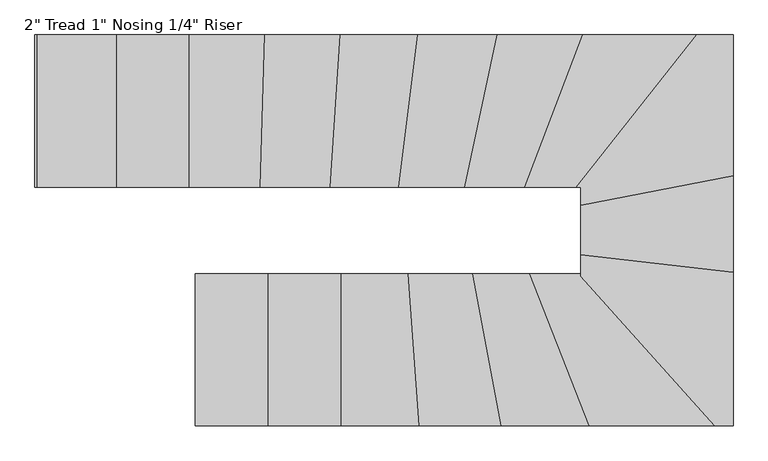
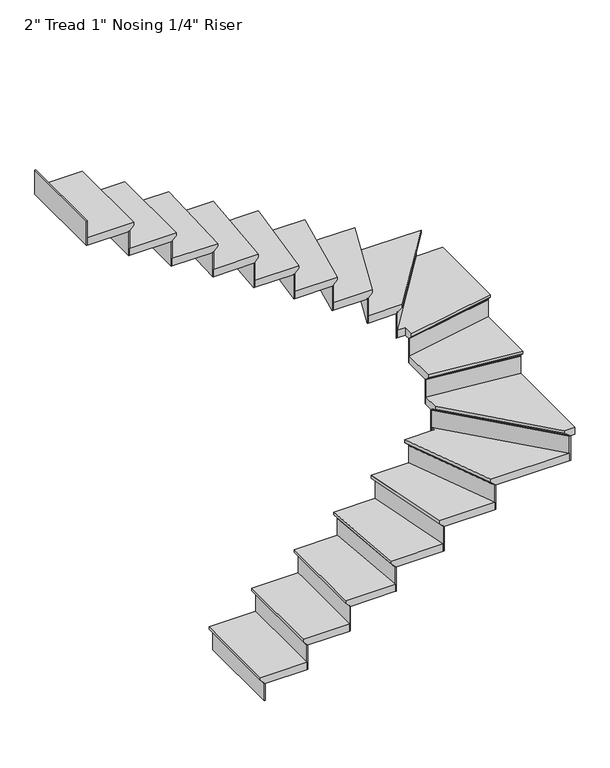
"""IFC4 building model written with IfcOpenShell, lengths in millimetres: stair flight geometry."""

from ifc_helpers import new_model, si_unit, origin, place, context, project, spatial, faceted_brep, source, transform, mapped, element, save


def stair_flight_08a12ea7(model_context):
    return source(origin(), model_context, "Body", "Brep", [
        faceted_brep([(376.3877765, 452.8595092, 150.2833333), (376.3877765, 452.8595092, 169.3333333), (376.3877765, 1037.0595092, 169.3333333), (376.3877765, 1037.0595092, 150.2833333), (401.7877765, 452.8595092, 124.8833333), (401.7877765, 1037.0595092, 124.8833333), (681.1877765, 452.8595092, 169.3333333), (681.1877765, 1037.0595092, 169.3333333), (401.7877765, 1037.0595092, 118.5333333), (681.1877765, 1037.0595092, 118.5333333), (681.1877765, 452.8595092, 118.5333333), (401.7877765, 452.8595092, 118.5333333)], [[[0, 1, 2, 3]], [[4, 0, 3, 5]], [[2, 1, 6, 7]], [[8, 9, 10, 11]], [[2, 7, 9, 8, 5, 3]], [[8, 11, 4, 5]], [[6, 1, 0, 4, 11, 10]], [[7, 6, 10, 9]]]),
        faceted_brep([(401.7877765, 452.8595092, 118.5333333), (401.7877765, 452.8595092, 0.0), (408.1377765, 452.8595092, 0.0), (408.1377765, 452.8595092, 118.5333333), (401.7877765, 1037.0595092, 118.5333333), (408.1377765, 1037.0595092, 118.5333333), (408.1377765, 1037.0595092, 0.0), (401.7877765, 1037.0595092, 0.0)], [[[0, 1, 2, 3]], [[4, 5, 6, 7]], [[1, 0, 4, 7]], [[2, 1, 7, 6]], [[3, 2, 6, 5]], [[0, 3, 5, 4]]]),
        faceted_brep([(681.1877765, 452.8595092, 287.8666667), (681.1877765, 452.8595092, 118.5333333), (687.5377765, 452.8595092, 118.5333333), (687.5377765, 452.8595092, 287.8666667), (681.1877765, 1037.0595092, 287.8666667), (687.5377765, 1037.0595092, 287.8666667), (687.5377765, 1037.0595092, 118.5333333), (681.1877765, 1037.0595092, 118.5333333)], [[[0, 1, 2, 3]], [[4, 5, 6, 7]], [[1, 0, 4, 7]], [[2, 1, 7, 6]], [[3, 2, 6, 5]], [[0, 3, 5, 4]]]),
        faceted_brep([(655.7877765, 1037.0595092, 338.6666667), (655.7877765, 452.8595092, 338.6666667), (960.5877765, 452.8595092, 338.6666667), (960.5877765, 1037.0595092, 338.6666667), (681.1877765, 1037.0595092, 287.8666667), (960.5877765, 1037.0595092, 287.8666667), (960.5877765, 452.8595092, 287.8666667), (681.1877765, 452.8595092, 287.8666667), (681.1877765, 1037.0595092, 294.2166667), (655.7877765, 1037.0595092, 319.6166667), (681.1877765, 452.8595092, 294.2166667), (655.7877765, 452.8595092, 319.6166667)], [[[0, 1, 2, 3]], [[4, 5, 6, 7]], [[0, 3, 5, 4, 8, 9]], [[4, 7, 10, 8]], [[2, 1, 11, 10, 7, 6]], [[3, 2, 6, 5]], [[11, 1, 0, 9]], [[10, 11, 9, 8]]]),
        faceted_brep([(960.5877765, 452.8595092, 457.2), (960.5877765, 452.8595092, 287.8666667), (966.9377765, 452.8595092, 287.8666667), (966.9377765, 452.8595092, 457.2), (960.5877765, 1037.0595092, 457.2), (966.9377765, 1037.0595092, 457.2), (966.9377765, 1037.0595092, 287.8666667), (960.5877765, 1037.0595092, 287.8666667)], [[[0, 1, 2, 3]], [[4, 5, 6, 7]], [[1, 0, 4, 7]], [[2, 1, 7, 6]], [[3, 2, 6, 5]], [[0, 3, 5, 4]]]),
        faceted_brep([(935.1877765, 1037.0595092, 508.0), (935.1877765, 452.8595092, 508.0), (1261.3926035, 452.8595092, 508.0), (1218.7183017, 1037.0595092, 508.0), (960.5877765, 1037.0595092, 457.2), (1218.7183017, 1037.0595092, 457.2), (1261.3926035, 452.8595092, 457.2), (960.5877765, 452.8595092, 457.2), (960.5877765, 1037.0595092, 463.55), (935.1877765, 1037.0595092, 488.95), (960.5877765, 452.8595092, 463.55), (935.1877765, 452.8595092, 488.95)], [[[0, 1, 2, 3]], [[4, 5, 6, 7]], [[0, 3, 5, 4, 8, 9]], [[4, 7, 10, 8]], [[2, 1, 11, 10, 7, 6]], [[3, 2, 6, 5]], [[11, 1, 0, 9]], [[10, 11, 9, 8]]]),
        faceted_brep([(1261.3926035, 452.8595092, 626.5333333), (1261.3926035, 452.8595092, 457.2), (1267.7595225, 452.8595092, 457.2), (1267.7595225, 452.8595092, 626.5333333), (1218.7183017, 1037.0595092, 626.5333333), (1225.0852207, 1037.0595092, 626.5333333), (1225.0852207, 1037.0595092, 457.2), (1218.7183017, 1037.0595092, 457.2)], [[[0, 1, 2, 3]], [[4, 5, 6, 7]], [[1, 0, 4, 7]], [[2, 1, 7, 6]], [[3, 2, 6, 5]], [[0, 3, 5, 4]]]),
        faceted_brep([(1193.2506256, 1037.0595092, 677.3333333), (1235.9249274, 452.8595092, 677.3333333), (1574.4949622, 452.8595092, 677.3333333), (1465.1625624, 1037.0595092, 677.3333333), (1218.7183017, 1037.0595092, 626.5333333), (1465.1625624, 1037.0595092, 626.5333333), (1574.4949622, 452.8595092, 626.5333333), (1261.3926035, 452.8595092, 626.5333333), (1218.7183017, 1037.0595092, 632.8833333), (1193.2506256, 1037.0595092, 658.2833333), (1261.3926035, 452.8595092, 632.8833333), (1235.9249274, 452.8595092, 658.2833333)], [[[0, 1, 2, 3]], [[4, 5, 6, 7]], [[0, 3, 5, 4, 8, 9]], [[4, 7, 10, 8]], [[2, 1, 11, 10, 7, 6]], [[3, 2, 6, 5]], [[11, 1, 0, 9]], [[10, 11, 9, 8]]]),
        faceted_brep([(1574.4949622, 452.8595092, 795.8666667), (1574.4949622, 452.8595092, 626.5333333), (1580.9552087, 452.8595092, 626.5333333), (1580.9552087, 452.8595092, 795.8666667), (1465.1625624, 1037.0595092, 795.8666667), (1471.6228089, 1037.0595092, 795.8666667), (1471.6228089, 1037.0595092, 626.5333333), (1465.1625624, 1037.0595092, 626.5333333)], [[[0, 1, 2, 3]], [[4, 5, 6, 7]], [[1, 0, 4, 7]], [[2, 1, 7, 6]], [[3, 2, 6, 5]], [[0, 3, 5, 4]]]),
        faceted_brep([(1439.3215766, 1037.0595092, 846.6666667), (1548.6539764, 452.8595092, 846.6666667), (1914.7030468, 452.8595092, 846.6666667), (1686.6073017, 1037.0595092, 846.6666667), (1465.1625624, 1037.0595092, 795.8666667), (1686.6073017, 1037.0595092, 795.8666667), (1914.7030468, 452.8595092, 795.8666667), (1574.4949622, 452.8595092, 795.8666667), (1465.1625624, 1037.0595092, 802.2166667), (1439.3215766, 1037.0595092, 827.6166667), (1574.4949622, 452.8595092, 802.2166667), (1548.6539764, 452.8595092, 827.6166667)], [[[0, 1, 2, 3]], [[4, 5, 6, 7]], [[0, 3, 5, 4, 8, 9]], [[4, 7, 10, 8]], [[2, 1, 11, 10, 7, 6]], [[3, 2, 6, 5]], [[11, 1, 0, 9]], [[10, 11, 9, 8]]]),
        faceted_brep([(1914.7030468, 452.8595092, 965.2), (1914.7030468, 452.8595092, 795.8666667), (1921.5198963, 452.8595092, 795.8666667), (1921.5198963, 452.8595092, 965.2), (1686.6073017, 1037.0595092, 965.2), (1693.4241511, 1037.0595092, 965.2), (1693.4241511, 1037.0595092, 795.8666667), (1686.6073017, 1037.0595092, 795.8666667)], [[[0, 1, 2, 3]], [[4, 5, 6, 7]], [[1, 0, 4, 7]], [[2, 1, 7, 6]], [[3, 2, 6, 5]], [[0, 3, 5, 4]]]),
        faceted_brep([(1854.0275323, 1065.0294947, 1016.0), (1854.0275323, 1037.0595092, 1016.0), (1659.3399039, 1037.0595092, 1016.0), (1887.4356491, 452.8595092, 1016.0), (2402.3959103, 452.8595092, 1016.0), (1854.0275323, 1037.0595092, 965.2), (1854.0275323, 1065.0294947, 965.2), (2402.3959103, 452.8595092, 965.2), (1914.7030468, 452.8595092, 965.2), (1686.6073017, 1037.0595092, 965.2), (1914.7030468, 452.8595092, 971.55), (1686.6073017, 1037.0595092, 971.55), (1887.4356491, 452.8595092, 996.95), (1659.3399039, 1037.0595092, 996.95)], [[[0, 1, 2, 3, 4]], [[5, 6, 7, 8, 9]], [[1, 0, 6, 5]], [[9, 8, 10, 11]], [[4, 3, 12, 10, 8, 7]], [[0, 4, 7, 6]], [[12, 3, 2, 13]], [[10, 12, 13, 11]], [[2, 1, 5, 9, 11, 13]]]),
        faceted_brep([(2402.3959103, 452.8595092, 1134.5333333), (2402.3959103, 452.8595092, 965.2), (2410.9210499, 452.8595092, 965.2), (2410.9210499, 452.8595092, 1134.5333333), (1854.0275323, 1065.0294947, 1134.5333333), (1854.0275323, 1074.546518, 1134.5333333), (1854.0275323, 1074.546518, 965.2), (1854.0275323, 1065.0294947, 965.2)], [[[0, 1, 2, 3]], [[4, 5, 6, 7]], [[1, 0, 4, 7]], [[2, 1, 7, 6]], [[3, 2, 6, 5]], [[0, 3, 5, 4]]]),
        faceted_brep([(1854.0275323, 1026.9614017, 1185.3333333), (2368.2953518, 452.8595092, 1185.3333333), (2438.2275323, 452.8595092, 1185.3333333), (2438.2275323, 1067.1925921, 1185.3333333), (1854.0275323, 1134.0548433, 1185.3333333), (1854.0275323, 1065.0294947, 1134.5333333), (1854.0275323, 1134.0548433, 1134.5333333), (2438.2275323, 1067.1925921, 1134.5333333), (2438.2275323, 452.8595092, 1134.5333333), (2402.3959103, 452.8595092, 1134.5333333), (1854.0275323, 1065.0294947, 1140.8833333), (1854.0275323, 1026.9614017, 1166.2833333), (2402.3959103, 452.8595092, 1140.8833333), (2368.2953518, 452.8595092, 1166.2833333)], [[[0, 1, 2, 3, 4]], [[5, 6, 7, 8, 9]], [[0, 4, 6, 5, 10, 11]], [[5, 9, 12, 10]], [[2, 1, 13, 12, 9, 8]], [[3, 2, 8, 7]], [[4, 3, 7, 6]], [[13, 1, 0, 11]], [[12, 13, 11, 10]]]),
        faceted_brep([(2438.2275323, 1067.1925921, 1303.8666667), (2438.2275323, 1067.1925921, 1134.5333333), (2438.2275323, 1073.5840462, 1134.5333333), (2438.2275323, 1073.5840462, 1303.8666667), (1854.0275323, 1134.0548433, 1303.8666667), (1854.0275323, 1140.4462974, 1303.8666667), (1854.0275323, 1140.4462974, 1134.5333333), (1854.0275323, 1134.0548433, 1134.5333333)], [[[0, 1, 2, 3]], [[4, 5, 6, 7]], [[1, 0, 4, 7]], [[2, 1, 7, 6]], [[3, 2, 6, 5]], [[0, 3, 5, 4]]]),
        faceted_brep([(1854.0275323, 1108.4890269, 1354.6666667), (2438.2275323, 1041.6267758, 1354.6666667), (2438.2275323, 1437.0400125, 1354.6666667), (1854.0275323, 1323.6242566, 1354.6666667), (1854.0275323, 1134.0548433, 1303.8666667), (1854.0275323, 1323.6242566, 1303.8666667), (2438.2275323, 1437.0400125, 1303.8666667), (2438.2275323, 1067.1925921, 1303.8666667), (1854.0275323, 1134.0548433, 1310.2166667), (1854.0275323, 1108.4890269, 1335.6166667), (2438.2275323, 1067.1925921, 1310.2166667), (2438.2275323, 1041.6267758, 1335.6166667)], [[[0, 1, 2, 3]], [[4, 5, 6, 7]], [[0, 3, 5, 4, 8, 9]], [[4, 7, 10, 8]], [[3, 2, 6, 5]], [[11, 1, 0, 9]], [[10, 11, 9, 8]], [[2, 1, 11, 10, 7, 6]]]),
        faceted_brep([(2438.2275323, 1437.0400125, 1473.2), (2438.2275323, 1437.0400125, 1303.8666667), (2438.2275323, 1443.5085708, 1303.8666667), (2438.2275323, 1443.5085708, 1473.2), (1854.0275323, 1323.6242566, 1473.2), (1854.0275323, 1330.0928149, 1473.2), (1854.0275323, 1330.0928149, 1303.8666667), (1854.0275323, 1323.6242566, 1303.8666667)], [[[0, 1, 2, 3]], [[4, 5, 6, 7]], [[1, 0, 4, 7]], [[2, 1, 7, 6]], [[3, 2, 6, 5]], [[0, 3, 5, 4]]]),
        faceted_brep([(1802.8941647, 1367.2595092, 1524.0), (1854.0275323, 1367.2595092, 1524.0), (1854.0275323, 1297.7500234, 1524.0), (2438.2275323, 1411.1657793, 1524.0), (2438.2275323, 1951.4595092, 1524.0), (2264.0560999, 1951.4595092, 1524.0), (1854.0275323, 1367.2595092, 1473.2), (1802.8941647, 1367.2595092, 1473.2), (2264.0560999, 1951.4595092, 1473.2), (2438.2275323, 1951.4595092, 1473.2), (2438.2275323, 1437.0400125, 1473.2), (1854.0275323, 1323.6242566, 1473.2), (2438.2275323, 1437.0400125, 1479.55), (1854.0275323, 1323.6242566, 1479.55), (2438.2275323, 1411.1657793, 1504.95), (1854.0275323, 1297.7500234, 1504.95)], [[[0, 1, 2, 3, 4, 5]], [[6, 7, 8, 9, 10, 11]], [[1, 0, 7, 6]], [[11, 10, 12, 13]], [[4, 3, 14, 12, 10, 9]], [[0, 5, 8, 7]], [[14, 3, 2, 15]], [[12, 14, 15, 13]], [[2, 1, 6, 11, 13, 15]], [[5, 4, 9, 8]]]),
        faceted_brep([(2264.0560999, 1951.4595092, 1642.5333333), (2264.0560999, 1951.4595092, 1473.2), (2255.966047, 1951.4595092, 1473.2), (2255.966047, 1951.4595092, 1642.5333333), (1802.8941647, 1367.2595092, 1642.5333333), (1794.8041118, 1367.2595092, 1642.5333333), (1794.8041118, 1367.2595092, 1473.2), (1802.8941647, 1367.2595092, 1473.2)], [[[0, 1, 2, 3]], [[4, 5, 6, 7]], [[1, 0, 4, 7]], [[2, 1, 7, 6]], [[3, 2, 6, 5]], [[0, 3, 5, 4]]]),
        faceted_brep([(1835.2543766, 1367.2595092, 1693.3333333), (2296.4163117, 1951.4595092, 1693.3333333), (1832.5459554, 1951.4595092, 1693.3333333), (1611.2993582, 1367.2595092, 1693.3333333), (1802.8941647, 1367.2595092, 1642.5333333), (1611.2993582, 1367.2595092, 1642.5333333), (1832.5459554, 1951.4595092, 1642.5333333), (2264.0560999, 1951.4595092, 1642.5333333), (1802.8941647, 1367.2595092, 1648.8833333), (1835.2543766, 1367.2595092, 1674.2833333), (2264.0560999, 1951.4595092, 1648.8833333), (2296.4163117, 1951.4595092, 1674.2833333)], [[[0, 1, 2, 3]], [[4, 5, 6, 7]], [[0, 3, 5, 4, 8, 9]], [[4, 7, 10, 8]], [[2, 1, 11, 10, 7, 6]], [[3, 2, 6, 5]], [[11, 1, 0, 9]], [[10, 11, 9, 8]]]),
        faceted_brep([(1832.5459554, 1951.4595092, 1811.8666667), (1832.5459554, 1951.4595092, 1642.5333333), (1825.7558284, 1951.4595092, 1642.5333333), (1825.7558284, 1951.4595092, 1811.8666667), (1611.2993582, 1367.2595092, 1811.8666667), (1604.5092312, 1367.2595092, 1811.8666667), (1604.5092312, 1367.2595092, 1642.5333333), (1611.2993582, 1367.2595092, 1642.5333333)], [[[0, 1, 2, 3]], [[4, 5, 6, 7]], [[1, 0, 4, 7]], [[2, 1, 7, 6]], [[3, 2, 6, 5]], [[0, 3, 5, 4]]]),
        faceted_brep([(1638.4598661, 1367.2595092, 1862.6666667), (1859.7064633, 1951.4595092, 1862.6666667), (1506.4045878, 1951.4595092, 1862.6666667), (1381.0045978, 1367.2595092, 1862.6666667), (1611.2993582, 1367.2595092, 1811.8666667), (1381.0045978, 1367.2595092, 1811.8666667), (1506.4045878, 1951.4595092, 1811.8666667), (1832.5459554, 1951.4595092, 1811.8666667), (1611.2993582, 1367.2595092, 1818.2166667), (1638.4598661, 1367.2595092, 1843.6166667), (1832.5459554, 1951.4595092, 1818.2166667), (1859.7064633, 1951.4595092, 1843.6166667)], [[[0, 1, 2, 3]], [[4, 5, 6, 7]], [[0, 3, 5, 4, 8, 9]], [[4, 7, 10, 8]], [[2, 1, 11, 10, 7, 6]], [[3, 2, 6, 5]], [[11, 1, 0, 9]], [[10, 11, 9, 8]]]),
        faceted_brep([(1506.4045878, 1951.4595092, 1981.2), (1506.4045878, 1951.4595092, 1811.8666667), (1499.9099448, 1951.4595092, 1811.8666667), (1499.9099448, 1951.4595092, 1981.2), (1381.0045978, 1367.2595092, 1981.2), (1374.5099549, 1367.2595092, 1981.2), (1374.5099549, 1367.2595092, 1811.8666667), (1381.0045978, 1367.2595092, 1811.8666667)], [[[0, 1, 2, 3]], [[4, 5, 6, 7]], [[1, 0, 4, 7]], [[2, 1, 7, 6]], [[3, 2, 6, 5]], [[0, 3, 5, 4]]]),
        faceted_brep([(1406.9831697, 1367.2595092, 2032.0), (1532.3831596, 1951.4595092, 2032.0), (1201.0973281, 1951.4595092, 2032.0), (1128.2758567, 1367.2595092, 2032.0), (1381.0045978, 1367.2595092, 1981.2), (1128.2758567, 1367.2595092, 1981.2), (1201.0973281, 1951.4595092, 1981.2), (1506.4045878, 1951.4595092, 1981.2), (1381.0045978, 1367.2595092, 1987.55), (1406.9831697, 1367.2595092, 2012.95), (1506.4045878, 1951.4595092, 1987.55), (1532.3831596, 1951.4595092, 2012.95)], [[[0, 1, 2, 3]], [[4, 5, 6, 7]], [[0, 3, 5, 4, 8, 9]], [[4, 7, 10, 8]], [[2, 1, 11, 10, 7, 6]], [[3, 2, 6, 5]], [[11, 1, 0, 9]], [[10, 11, 9, 8]]]),
        faceted_brep([(1201.0973281, 1951.4595092, 2150.5333333), (1201.0973281, 1951.4595092, 1981.2), (1194.6981851, 1951.4595092, 1981.2), (1194.6981851, 1951.4595092, 2150.5333333), (1128.2758567, 1367.2595092, 2150.5333333), (1121.8767136, 1367.2595092, 2150.5333333), (1121.8767136, 1367.2595092, 1981.2), (1128.2758567, 1367.2595092, 1981.2)], [[[0, 1, 2, 3]], [[4, 5, 6, 7]], [[1, 0, 4, 7]], [[2, 1, 7, 6]], [[3, 2, 6, 5]], [[0, 3, 5, 4]]]),
        faceted_brep([(1153.8724289, 1367.2595092, 2201.3333333), (1226.6939004, 1951.4595092, 2201.3333333), (905.2286579, 1951.4595092, 2201.3333333), (865.6210523, 1367.2595092, 2201.3333333), (1128.2758567, 1367.2595092, 2150.5333333), (865.6210523, 1367.2595092, 2150.5333333), (905.2286579, 1951.4595092, 2150.5333333), (1201.0973281, 1951.4595092, 2150.5333333), (1128.2758567, 1367.2595092, 2156.8833333), (1153.8724289, 1367.2595092, 2182.2833333), (1201.0973281, 1951.4595092, 2156.8833333), (1226.6939004, 1951.4595092, 2182.2833333)], [[[0, 1, 2, 3]], [[4, 5, 6, 7]], [[0, 3, 5, 4, 8, 9]], [[4, 7, 10, 8]], [[2, 1, 11, 10, 7, 6]], [[3, 2, 6, 5]], [[11, 1, 0, 9]], [[10, 11, 9, 8]]]),
        faceted_brep([(905.2286579, 1951.4595092, 2319.8666667), (905.2286579, 1951.4595092, 2150.5333333), (898.8640805, 1951.4595092, 2150.5333333), (898.8640805, 1951.4595092, 2319.8666667), (865.6210523, 1367.2595092, 2319.8666667), (859.2564749, 1367.2595092, 2319.8666667), (859.2564749, 1367.2595092, 2150.5333333), (865.6210523, 1367.2595092, 2150.5333333)], [[[0, 1, 2, 3]], [[4, 5, 6, 7]], [[1, 0, 4, 7]], [[2, 1, 7, 6]], [[3, 2, 6, 5]], [[0, 3, 5, 4]]]),
        faceted_brep([(891.0793619, 1367.2595092, 2370.6666667), (930.6869675, 1951.4595092, 2370.6666667), (614.4347929, 1951.4595092, 2370.6666667), (597.7107248, 1367.2595092, 2370.6666667), (865.6210523, 1367.2595092, 2319.8666667), (597.7107248, 1367.2595092, 2319.8666667), (614.4347929, 1951.4595092, 2319.8666667), (905.2286579, 1951.4595092, 2319.8666667), (865.6210523, 1367.2595092, 2326.2166667), (891.0793619, 1367.2595092, 2351.6166667), (905.2286579, 1951.4595092, 2326.2166667), (930.6869675, 1951.4595092, 2351.6166667)], [[[0, 1, 2, 3]], [[4, 5, 6, 7]], [[0, 3, 5, 4, 8, 9]], [[4, 7, 10, 8]], [[2, 1, 11, 10, 7, 6]], [[3, 2, 6, 5]], [[11, 1, 0, 9]], [[10, 11, 9, 8]]]),
        faceted_brep([(614.4347929, 1951.4595092, 2489.2), (614.4347929, 1951.4595092, 2319.8666667), (608.0821915, 1951.4595092, 2319.8666667), (608.0821915, 1951.4595092, 2489.2), (597.7107248, 1367.2595092, 2489.2), (591.3581233, 1367.2595092, 2489.2), (591.3581233, 1367.2595092, 2319.8666667), (597.7107248, 1367.2595092, 2319.8666667)], [[[0, 1, 2, 3]], [[4, 5, 6, 7]], [[1, 0, 4, 7]], [[2, 1, 7, 6]], [[3, 2, 6, 5]], [[0, 3, 5, 4]]]),
        faceted_brep([(623.1211306, 1367.2595092, 2540.0), (639.8451987, 1951.4595092, 2540.0), (326.6831647, 1951.4595092, 2540.0), (326.6831647, 1367.2595092, 2540.0), (597.7107248, 1367.2595092, 2489.2), (326.6831647, 1367.2595092, 2489.2), (326.6831647, 1951.4595092, 2489.2), (614.4347929, 1951.4595092, 2489.2), (597.7107248, 1367.2595092, 2495.55), (623.1211306, 1367.2595092, 2520.95), (614.4347929, 1951.4595092, 2495.55), (639.8451987, 1951.4595092, 2520.95)], [[[0, 1, 2, 3]], [[4, 5, 6, 7]], [[0, 3, 5, 4, 8, 9]], [[4, 7, 10, 8]], [[2, 1, 11, 10, 7, 6]], [[3, 2, 6, 5]], [[11, 1, 0, 9]], [[10, 11, 9, 8]]]),
        faceted_brep([(326.6831647, 1951.4595092, 2658.5333333), (326.6831647, 1951.4595092, 2489.2), (320.3331647, 1951.4595092, 2489.2), (320.3331647, 1951.4595092, 2658.5333333), (326.6831647, 1367.2595092, 2658.5333333), (320.3331647, 1367.2595092, 2658.5333333), (320.3331647, 1367.2595092, 2489.2), (326.6831647, 1367.2595092, 2489.2)], [[[0, 1, 2, 3]], [[4, 5, 6, 7]], [[1, 0, 4, 7]], [[2, 1, 7, 6]], [[3, 2, 6, 5]], [[0, 3, 5, 4]]]),
        faceted_brep([(352.0831647, 1367.2595092, 2709.3333333), (352.0831647, 1951.4595092, 2709.3333333), (47.2831647, 1951.4595092, 2709.3333333), (47.2831647, 1367.2595092, 2709.3333333), (326.6831647, 1367.2595092, 2658.5333333), (47.2831647, 1367.2595092, 2658.5333333), (47.2831647, 1951.4595092, 2658.5333333), (326.6831647, 1951.4595092, 2658.5333333), (326.6831647, 1367.2595092, 2664.8833333), (352.0831647, 1367.2595092, 2690.2833333), (326.6831647, 1951.4595092, 2664.8833333), (352.0831647, 1951.4595092, 2690.2833333)], [[[0, 1, 2, 3]], [[4, 5, 6, 7]], [[0, 3, 5, 4, 8, 9]], [[4, 7, 10, 8]], [[2, 1, 11, 10, 7, 6]], [[3, 2, 6, 5]], [[11, 1, 0, 9]], [[10, 11, 9, 8]]]),
        faceted_brep([(47.2831647, 1951.4595092, 2827.8666667), (47.2831647, 1951.4595092, 2658.5333333), (40.9331647, 1951.4595092, 2658.5333333), (40.9331647, 1951.4595092, 2827.8666667), (47.2831647, 1367.2595092, 2827.8666667), (40.9331647, 1367.2595092, 2827.8666667), (40.9331647, 1367.2595092, 2658.5333333), (47.2831647, 1367.2595092, 2658.5333333)], [[[0, 1, 2, 3]], [[4, 5, 6, 7]], [[1, 0, 4, 7]], [[2, 1, 7, 6]], [[3, 2, 6, 5]], [[0, 3, 5, 4]]]),
        faceted_brep([(-232.1168353, 1951.4595092, 2997.2), (-232.1168353, 1951.4595092, 2827.8666667), (-238.4668353, 1951.4595092, 2827.8666667), (-238.4668353, 1951.4595092, 2997.2), (-232.1168353, 1367.2595092, 2997.2), (-238.4668353, 1367.2595092, 2997.2), (-238.4668353, 1367.2595092, 2827.8666667), (-232.1168353, 1367.2595092, 2827.8666667)], [[[0, 1, 2, 3]], [[4, 5, 6, 7]], [[1, 0, 4, 7]], [[2, 1, 7, 6]], [[3, 2, 6, 5]], [[0, 3, 5, 4]]]),
        faceted_brep([(72.6831647, 1367.2595092, 2878.6666667), (72.6831647, 1951.4595092, 2878.6666667), (-232.1168353, 1951.4595092, 2878.6666667), (-232.1168353, 1367.2595092, 2878.6666667), (47.2831647, 1367.2595092, 2827.8666667), (-232.1168353, 1367.2595092, 2827.8666667), (-232.1168353, 1951.4595092, 2827.8666667), (47.2831647, 1951.4595092, 2827.8666667), (47.2831647, 1367.2595092, 2834.2166667), (72.6831647, 1367.2595092, 2859.6166667), (47.2831647, 1951.4595092, 2834.2166667), (72.6831647, 1951.4595092, 2859.6166667)], [[[0, 1, 2, 3]], [[4, 5, 6, 7]], [[0, 3, 5, 4, 8, 9]], [[4, 7, 10, 8]], [[2, 1, 11, 10, 7, 6]], [[3, 2, 6, 5]], [[11, 1, 0, 9]], [[10, 11, 9, 8]]]),
    ])


if __name__ == "__main__":
    model = new_model("IFC4")
    model_context = context("Model", 3, world=origin())
    ifc_project = project(units=[si_unit("LENGTHUNIT", "METRE", prefix="MILLI")], contexts=[model_context])
    site = spatial("IfcSite", under=ifc_project)
    building = spatial("IfcBuilding", under=site)
    placement = place(None, origin())
    stair_flight_shape = stair_flight_08a12ea7(model_context)
    element("IfcStairFlight", 1, ObjectType="2\" Tread 1\" Nosing 1/4\" Riser", at=placement, inside=building, context=model_context, shape_type="MappedRepresentation", body=[
        mapped(stair_flight_shape, transform((0.0, 0.0, 0.0), x_axis=(1.0, 0.0, 0.0), y_axis=(0.0, 1.0, 0.0), z_axis=(0.0, 0.0, 1.0))),
    ])
    save(model, "model.ifc")
